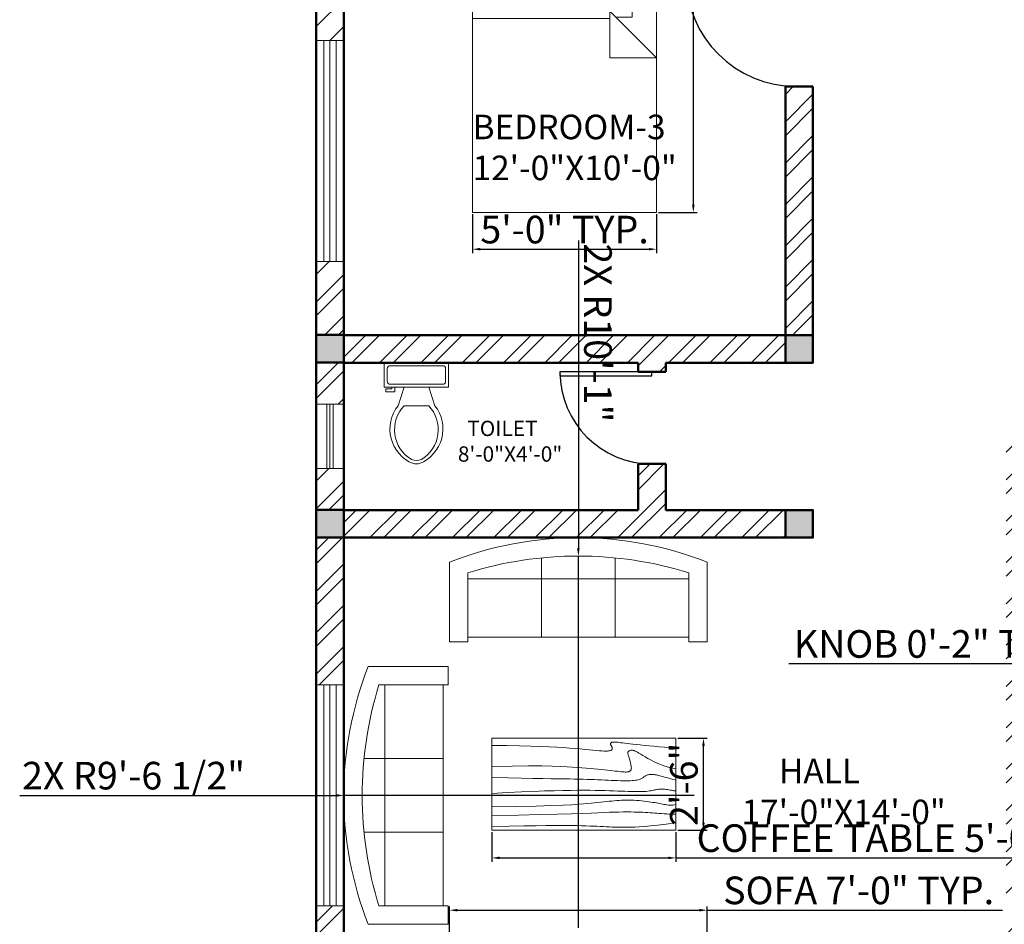
# Model space of a CAD drawing. Units: inches. Extents: x 381 to 1001, y 3003 to 3971.
# Tile 2 of 4: x 381 to 702, y 3347 to 3641. Entities that reach past the tile are written whole.
import ezdxf

# ---------------------------------------------------------------- set-up
doc = ezdxf.new("R2010")
doc.units = ezdxf.units.IN
for name, color, linetype, lineweight in [('A-ANNO-DIMS', 2, 'Continuous', 18), ('A-AREA-IDEN', 7, 'Continuous', 18), ('A-COLS', 7, 'Continuous', 50), ('A-DOOR', 4, 'Continuous', 25), ('A-FLOR-FIXT', 9, 'Continuous', 18), ('A-FURN', 8, 'Continuous', 18), ('A-GLAZ', 244, 'Continuous', 18), ('A-WALL', 7, 'Continuous', 50), ('A-WALL-PATT', 252, 'Continuous', 13)]:
    doc.layers.add(name, color=color, linetype=linetype, lineweight=lineweight)
doc.styles.get("Standard").update_dxf_attribs({"font": 'arial.ttf'})
doc.dimstyles.new('ISO-25', dxfattribs={"dimtxt": 9, "dimasz": 2.5, "dimexe": 1.25, "dimexo": 0.625, "dimtad": 1, "dimlunit": 3, "dimtxsty": 'Standard', "dimcen": 2.5, "dimadec": 0, "dimazin": 0, "dimtfac": 1, "dimtmove": 0, "dimatfit": 3, "dimfxl": 1, "dimarcsym": 0})

# ---------------------------------------------------------------- blocks, each defined once
blk = doc.blocks.new('*U3')
for p, q in [((0, 0), (0, -6)), ((-40, 0), (-40, -6))]:
    blk.add_line(p, q)
blk.add_lwpolyline([(0, 0), (0, 40), (-1.75, 40), (-1.75, 0)], close=True)
blk.add_arc((0, 0), 40, 90, 180)
blk = doc.blocks.new('*U9')
for p, q in [((9.5, -6), (9.5, -2)), ((-10, -8.5), (-8, -8.5)), ((-10, -9.5), (-10, -8.5)), ((-7, -9.5), (-10, -9.5)), ((-8, -8.5), (-8, -8)), ((-7, -8), (-7, -9.5)), ((-4, -8), (-6, -14)), ((4, -8), (6, -14)), ((4, -14), (-4, -14))]:
    blk.add_line(p, q)
blk.add_lwpolyline([(10.5, -8), (10.5, 0), (-10.5, 0), (-10.5, -8)], close=True)
for points in [[(-9.5, -2), (-9.5, -6)], [(8.5, -1), (-8.5, -1)], [(-8.5, -7), (8.5, -7)]]:
    blk.add_lwpolyline(points)
for centre, radius, start, end in [((-8.62, -1.88), 0.884, 81.8699, 188.1301), ((8.62, -1.88), 0.884, 351.8699, 98.1301), ((-8.62, -6.12), 0.884, 171.8699, 278.1301), ((8.62, -6.12), 0.884, 261.8699, 8.1301), ((3.52, -21.58), 12.17, 141.4691, 247.9714), ((4.2, -21.82), 11.33, 136.3677, 238.9468), ((-3.52, -21.58), 12.17, 292.0284, 38.5307), ((-4.2, -21.82), 11.33, 301.053, 43.6321), ((0, -27.88), 4, 245.7318, 294.2682), ((0, -29), 4, 254.8605, 285.1395)]:
    blk.add_arc(centre, radius, start, end)
blk = doc.blocks.new('Bed - Queen')
for p, q in [((0, -80.00003), (0, 0)), ((0, 0), (59.99999, 0)), ((59.99999, 0), (59.99999, -80.00003)), ((7.99999, -1.2), (28.79998, -1.2)), ((7.99999, -14.4), (7.99999, -1.2)), ((28.79998, -1.2), (28.79998, -14.4)), ((31.19999, -1.2), (51.99999, -1.2)), ((31.19999, -14.4), (31.19999, -1.2)), ((51.99999, -1.2), (51.99999, -16.4)), ((0, -14.4), (44.8, -14.4)), ((59.99999, -29.6), (44.8, -14.4)), ((44.8, -14.4), (44.8, -29.6)), ((44.8, -16.8), (0, -16.8)), ((51.99999, -16.4), (46.79936, -16.4)), ((44.8, -29.6), (59.99999, -29.6)), ((59.99999, -80.00003), (0, -80.00003))]:
    blk.add_line(p, q)
blk = doc.blocks.new('Sofa - Roundback 7 ft.')
for p, q in [((-12.00002, -32.4421), (-12.00003, -6.5971)), ((11.99997, -32.4421), (11.99998, -6.5971)), ((-36.000027, -34), (-36.000027, -11.4696)), ((35.99998, -34), (35.99998, -11.4696)), ((-35.999844, -13.3819), (35.9998, -13.3819)), ((-36.000027, -32.4421), (35.99998, -32.4421))]:
    blk.add_line(p, q)
for points in [[(-36.000027, -34), (-42.000027, -34), (-42.000027, -8)], [(41.99998, -8), (41.99998, -34), (35.99998, -34)]]:
    blk.add_lwpolyline(points)
for centre, radius, start, end in [((0, -114.25), 114.25, 68.43141, 111.5686), ((-0.00001, -127.1968), 121.1968, 72.72033, 107.2797)]:
    blk.add_arc(centre, radius, start, end)
blk = doc.blocks.new('Table - Rectangular Woodgrain 60 x 30 in.')
for p, q in [((0, 0), (0, -30)), ((60, 0), (0, 0)), ((60, -30), (60, 0)), ((0, -30), (60, -30))]:
    blk.add_line(p, q)
for points in [[(0, -2.4), (4.8155, -2.418), (9.0302, -2.4688), (12.709, -2.5477), (15.9167, -2.65), (18.7181, -2.7711), (21.1781, -2.9063), (23.3616, -3.0508), (25.3333, -3.2), (27.1477, -3.3495), (28.8172, -3.4958), (30.3437, -3.636), (31.7291, -3.7667), (32.9756, -3.8849), (34.0849, -3.9875), (35.059, -4.0714), (35.9, -4.1334), (36.6114, -4.1711), (37.2041, -4.1854), (37.6906, -4.1779), (38.0833, -4.15), (38.3948, -4.1034), (38.6375, -4.0396), (38.8239, -3.9602), (38.9666, -3.8667), (39.0764, -3.7608), (39.1573, -3.6448), (39.2116, -3.521), (39.2416, -3.3917), (39.2498, -3.2593), (39.2385, -3.1261), (39.21, -2.9944), (39.1666, -2.8667), (39.111, -2.7447), (39.0468, -2.6281), (38.978, -2.5163), (38.9083, -2.4083), (38.8418, -2.3035), (38.7823, -2.201), (38.7337, -2.1001), (38.7, -2), (38.6844, -1.9003), (38.6875, -1.8021), (38.7094, -1.707), (38.75, -1.6167), (38.8094, -1.5326), (38.8875, -1.4563), (38.9844, -1.3893), (39.1, -1.3333), (39.2351, -1.2896), (39.3937, -1.2583), (39.5804, -1.2396), (39.8, -1.2333), (40.057, -1.2396), (40.3562, -1.2583), (40.7023, -1.2896), (41.1, -1.3333), (41.5547, -1.3895), (42.0755, -1.4573), (42.6721, -1.5361), (43.3542, -1.625), (44.1316, -1.7233), (45.014, -1.8302), (46.0114, -1.9449), (47.1333, -2.0667), (48.3862, -2.1947), (49.7625, -2.3281), (51.2513, -2.4663), (52.8416, -2.6083), (54.5226, -2.7535), (56.2833, -2.9011), (58.1127, -3.0501), (60, -3.2)], [(0, -9.2), (6.5759, -9.0858), (11.9385, -9.0365), (16.2527, -9.0418), (19.6833, -9.0917), (22.3952, -9.1759), (24.5531, -9.2844), (26.322, -9.4069), (27.8666, -9.5333), (29.3241, -9.6553), (30.7203, -9.7719), (32.0532, -9.8837), (33.3208, -9.9917), (34.5213, -10.0965), (35.6526, -10.199), (36.7128, -10.2999), (37.7, -10.4), (38.6129, -10.4996), (39.4531, -10.5969), (40.223, -10.6895), (40.925, -10.775), (41.5613, -10.8512), (42.1344, -10.9156), (42.6465, -10.966), (43.1, -11), (43.4976, -11.0158), (43.8437, -11.0136), (44.143, -10.9942), (44.4, -10.9583), (44.6195, -10.9069), (44.8062, -10.8406), (44.9648, -10.7603), (45.1, -10.6667), (45.2155, -10.5598), (45.3114, -10.4365), (45.3871, -10.2929), (45.4416, -10.125), (45.4743, -9.929), (45.4844, -9.7011), (45.4709, -9.4371), (45.4333, -9.1333), (45.3716, -8.7883), (45.2896, -8.4104), (45.1919, -8.0107), (45.0833, -7.6), (44.9685, -7.1893), (44.8521, -6.7896), (44.7388, -6.4117), (44.6333, -6.0667), (44.54, -5.7628), (44.4614, -5.4979), (44.4001, -5.2675), (44.3583, -5.0667), (44.3384, -4.8909), (44.3427, -4.7354), (44.3736, -4.5956), (44.4333, -4.4667), (44.5236, -4.3453), (44.6427, -4.2333), (44.7884, -4.1339), (44.9583, -4.05), (45.1501, -3.9849), (45.3614, -3.9417), (45.59, -3.9234), (45.8333, -3.9333), (46.0915, -3.9749), (46.3734, -4.0531), (46.6906, -4.1736), (47.0542, -4.3417), (47.4756, -4.5629), (47.9661, -4.8427), (48.5372, -5.1866), (49.2, -5.6), (49.9676, -6.0844), (50.8594, -6.625), (51.8965, -7.2031), (53.1, -7.8), (54.491, -8.3969), (56.0906, -8.975), (57.9199, -9.5156), (60, -10)], [(0, -12.8), (5.1847, -12.9322), (9.6213, -13.0323), (13.3963, -13.1059), (16.5958, -13.1583), (19.3063, -13.1952), (21.614, -13.2219), (23.6054, -13.2439), (25.3666, -13.2667), (26.9728, -13.2947), (28.4531, -13.3281), (29.8256, -13.3663), (31.1083, -13.4083), (32.3191, -13.4535), (33.476, -13.501), (34.597, -13.5501), (35.7, -13.6), (36.7984, -13.6497), (37.8875, -13.6979), (38.9578, -13.743), (40, -13.7833), (41.0047, -13.8174), (41.9625, -13.8438), (42.864, -13.8607), (43.7, -13.8667), (44.4631, -13.8604), (45.1552, -13.8417), (45.7801, -13.8104), (46.3416, -13.7667), (46.8439, -13.7104), (47.2906, -13.6417), (47.6858, -13.5604), (48.0333, -13.4667), (48.3375, -13.3608), (48.6042, -13.2448), (48.8396, -13.121), (49.05, -12.9917), (49.2417, -12.8593), (49.4208, -12.7261), (49.5937, -12.5944), (49.7667, -12.4667), (49.9452, -12.3451), (50.1323, -12.2313), (50.3303, -12.1268), (50.5416, -12.0333), (50.7686, -11.9524), (51.0135, -11.8854), (51.2788, -11.8341), (51.5666, -11.8), (51.8785, -11.7843), (52.2116, -11.7865), (52.562, -11.8059), (52.926, -11.8417), (53.2998, -11.8931), (53.6795, -11.9594), (54.0614, -12.0397), (54.4416, -12.1333), (54.8223, -12.2401), (55.2293, -12.3625), (55.6942, -12.5037), (56.2489, -12.6667), (56.9251, -12.8547), (57.7545, -13.0708), (58.7689, -13.3182), (60, -13.6)], [(0, -18), (5.124, -17.7273), (9.6609, -17.5057), (13.6705, -17.3303), (17.2125, -17.1958), (20.3467, -17.0973), (23.1328, -17.0297), (25.6307, -16.9878), (27.9, -16.9667), (29.9928, -16.9617), (31.9302, -16.9703), (33.7254, -16.9907), (35.3917, -17.0208), (36.9423, -17.0588), (38.3906, -17.1026), (39.7499, -17.1503), (41.0333, -17.2), (42.2519, -17.2496), (43.4073, -17.2969), (44.4986, -17.3395), (45.525, -17.375), (46.4858, -17.4012), (47.3802, -17.4156), (48.2074, -17.416), (48.9667, -17.4), (49.6583, -17.3662), (50.2872, -17.3167), (50.8595, -17.2547), (51.3812, -17.1833), (51.8584, -17.1057), (52.2971, -17.025), (52.7034, -16.9443), (53.0833, -16.8667), (53.443, -16.7951), (53.789, -16.7313), (54.128, -16.6768), (54.4666, -16.6334), (54.8115, -16.6024), (55.1693, -16.5854), (55.5465, -16.5841), (55.95, -16.6), (56.3828, -16.6337), (56.8346, -16.6823), (57.2915, -16.7418), (57.7396, -16.8084), (58.165, -16.878), (58.5539, -16.9469), (58.8924, -17.0111), (59.1666, -17.0667), (59.3679, -17.1107), (59.5078, -17.1438), (59.6032, -17.1675), (59.6708, -17.1833), (59.7275, -17.193), (59.7901, -17.1979), (59.8753, -17.1998), (60, -17.2)], [(0, -22.4), (8.0098, -22.2501), (14.4094, -22.1011), (19.4168, -21.9535), (23.25, -21.8083), (26.1269, -21.6663), (28.2656, -21.5281), (29.884, -21.3947), (31.2, -21.2667), (32.3967, -21.1448), (33.5172, -21.0292), (34.5697, -20.9198), (35.5625, -20.8167), (36.5037, -20.7198), (37.4015, -20.6292), (38.2642, -20.5448), (39.1, -20.4667), (39.9164, -20.3951), (40.7187, -20.3313), (41.5117, -20.2768), (42.3, -20.2333), (43.0883, -20.2024), (43.8812, -20.1854), (44.6836, -20.1841), (45.5, -20.2), (46.3328, -20.234), (47.1747, -20.2844), (48.0163, -20.3488), (48.8479, -20.425), (49.66, -20.5106), (50.4429, -20.6031), (51.1872, -20.7004), (51.8833, -20.8), (52.5246, -20.8999), (53.1166, -20.9995), (53.6681, -21.0983), (54.1875, -21.1958), (54.6834, -21.2919), (55.1646, -21.3859), (55.6394, -21.4777), (56.1167, -21.5667), (56.6028, -21.6515), (57.0961, -21.7266), (57.5929, -21.7852), (58.0896, -21.8208), (58.5823, -21.8268), (59.0674, -21.7964), (59.5412, -21.723), (60, -21.6)], [(0, -25.2), (8.6355, -25.0504), (15.7026, -24.9031), (21.4049, -24.7606), (25.9458, -24.625), (29.529, -24.4988), (32.3578, -24.3844), (34.6359, -24.284), (36.5667, -24.2), (38.3213, -24.1341), (39.9417, -24.0854), (41.437, -24.0523), (42.8167, -24.0333), (44.0901, -24.0268), (45.2667, -24.0313), (46.3557, -24.0451), (47.3667, -24.0667), (48.309, -24.0947), (49.1928, -24.1287), (50.0284, -24.168), (50.826, -24.2125), (51.5959, -24.2617), (52.3483, -24.3151), (53.0935, -24.3725), (53.8417, -24.4334), (54.6009, -24.497), (55.3699, -24.561), (56.1454, -24.6226), (56.9239, -24.6792), (57.7021, -24.7279), (58.4764, -24.7662), (59.2435, -24.7911), (60, -24.8)], [(0, -28.8), (5.6867, -28.6681), (10.45, -28.5698), (14.407, -28.5012), (17.675, -28.4584), (20.3711, -28.4374), (22.6125, -28.4344), (24.5164, -28.4455), (26.2, -28.4667), (27.762, -28.4947), (29.2276, -28.5281), (30.6033, -28.5663), (31.8958, -28.6084), (33.1118, -28.6535), (34.2578, -28.7011), (35.3405, -28.7501), (36.3666, -28.8), (37.3443, -28.8497), (38.288, -28.8974), (39.2137, -28.9412), (40.1375, -28.9792), (41.0753, -29.0093), (42.0432, -29.0297), (43.0572, -29.0384), (44.1333, -29.0333), (45.2936, -29.0114), (46.5843, -28.9641), (48.0579, -28.8816), (49.7666, -28.7542), (51.7629, -28.5721), (54.0989, -28.3255), (56.8272, -28.0048), (60, -27.6)]]:
    blk.add_lwpolyline(points)
blk = doc.blocks.new('WIN-72X9')
for p, q in [((72, 6.5), (0, 6.5)), ((72, 4.5), (0, 4.5)), ((72, 2.5), (0, 2.5))]:
    blk.add_line(p, q)
blk.add_lwpolyline([(72, 9), (72, 0), (0, 0), (0, 9)], close=True)
blk = doc.blocks.new('VENT-WIN-21X9')
for p, q in [((3.5, 0), (3.5, 21)), ((4.5, 0), (4.5, 21)), ((5.5, 0), (5.5, 21))]:
    blk.add_line(p, q)
blk.add_lwpolyline([(9, 21), (9, 0), (0, 0), (0, 21)], close=True)
blk = doc.blocks.new('COLUMN-9X9')
h = blk.add_hatch(color=256)
h.dxf.hatch_style = 1
h.paths.add_polyline_path([(9, 9), (0, 9), (0, 0), (9, 0)])
blk.add_lwpolyline([(0, 9), (9, 9), (9, 0), (0, 0)], close=True)
blk = doc.blocks.new('*D36')
at = {"layer": 'A-ANNO-DIMS', "color": 0, "lineweight": -2, "transparency": 16777216}
for p, q in [((601.08, 3658.56), (601.08, 3794.71)), ((589.7, 3658.56), (602.33, 3658.56)), ((601.08, 3581.06), (601.08, 3656.06)), ((589.7, 3578.56), (602.33, 3578.56))]:
    blk.add_line(p, q, dxfattribs=at)
at = {"layer": 'A-ANNO-DIMS', "color": 0, "transparency": 16777216}
for points in [[(600.66, 3656.06), (601.49, 3656.06), (601.08, 3658.56)], [(600.66, 3581.06), (601.49, 3581.06), (601.08, 3578.56)]]:
    blk.add_solid(points, dxfattribs=at)
at = {"layer": 'Defpoints', "color": 0, "transparency": 16777216}
for p in [(589.08, 3658.56), (601.08, 3658.56), (589.08, 3578.56)]:
    blk.add_point(p, dxfattribs=at)
at = {"layer": 'A-ANNO-DIMS', "color": 0, "transparency": 16777216, "insert": (595.52, 3727.89), "char_height": 9, "attachment_point": 5, "rotation": 90}
blk.add_mtext('QUEEN BED 6\'-8" TYP.', dxfattribs=at)
blk = doc.blocks.new('*D37')
at = {"layer": 'A-ANNO-DIMS', "color": 0, "lineweight": -2, "transparency": 16777216}
for p, q in [((529.08, 3577.94), (529.08, 3565.31)), ((589.08, 3577.94), (589.08, 3565.31)), ((531.58, 3566.56), (586.58, 3566.56))]:
    blk.add_line(p, q, dxfattribs=at)
at = {"layer": 'A-ANNO-DIMS', "color": 0, "transparency": 16777216}
for points in [[(531.58, 3566.98), (531.58, 3566.15), (529.08, 3566.56)], [(586.58, 3566.98), (586.58, 3566.15), (589.08, 3566.56)]]:
    blk.add_solid(points, dxfattribs=at)
at = {"layer": 'Defpoints', "color": 0, "transparency": 16777216}
for p in [(529.08, 3578.56), (589.08, 3578.56), (589.08, 3566.56)]:
    blk.add_point(p, dxfattribs=at)
at = {"layer": 'A-ANNO-DIMS', "color": 0, "transparency": 16777216, "insert": (559.08, 3571.79), "char_height": 9, "attachment_point": 5}
blk.add_mtext('5\'-0" TYP.', dxfattribs=at)
blk = doc.blocks.new('*D38')
at = {"layer": 'A-ANNO-DIMS', "color": 0, "lineweight": -2, "transparency": 16777216}
for p, q in [((521.58, 3339.19), (521.58, 3352.41)), ((605.58, 3339.19), (605.58, 3352.41)), ((524.08, 3351.16), (603.08, 3351.16)), ((605.58, 3351.16), (701.87, 3351.16))]:
    blk.add_line(p, q, dxfattribs=at)
at = {"layer": 'A-ANNO-DIMS', "color": 0, "transparency": 16777216}
for points in [[(524.08, 3351.58), (524.08, 3350.75), (521.58, 3351.16)], [(603.08, 3351.58), (603.08, 3350.75), (605.58, 3351.16)]]:
    blk.add_solid(points, dxfattribs=at)
at = {"layer": 'Defpoints', "color": 0, "transparency": 16777216}
for p in [(605.58, 3351.16), (521.58, 3338.56), (605.58, 3338.56)]:
    blk.add_point(p, dxfattribs=at)
at = {"layer": 'A-ANNO-DIMS', "color": 0, "transparency": 16777216, "insert": (654.97, 3356.45), "char_height": 9, "attachment_point": 5}
blk.add_mtext('SOFA 7\'-0" TYP.', dxfattribs=at)
blk = doc.blocks.new('*D46')
at = {"layer": 'A-ANNO-DIMS', "color": 0, "lineweight": -2, "transparency": 16777216}
for p, q in [((732.1, 3431.81), (732.1, 3432.72)), ((733.98, 3431.81), (733.98, 3432.72)), ((729.6, 3431.47), (632.26, 3431.47)), ((733.98, 3431.47), (732.1, 3431.47)), ((736.48, 3431.47), (738.98, 3431.47))]:
    blk.add_line(p, q, dxfattribs=at)
at = {"layer": 'A-ANNO-DIMS', "color": 0, "transparency": 16777216}
for points in [[(729.6, 3431.88), (729.6, 3431.05), (732.1, 3431.47)], [(736.48, 3431.88), (736.48, 3431.05), (733.98, 3431.47)]]:
    blk.add_solid(points, dxfattribs=at)
at = {"layer": 'Defpoints', "color": 0, "transparency": 16777216}
for p in [(732.1, 3431.47), (732.1, 3431.18), (733.98, 3431.18)]:
    blk.add_point(p, dxfattribs=at)
at = {"layer": 'A-ANNO-DIMS', "color": 0, "transparency": 16777216, "insert": (679.68, 3436.75), "char_height": 9, "attachment_point": 5}
blk.add_mtext('KNOB 0\'-2" TYP.', dxfattribs=at)
blk = doc.blocks.new('*D50')
at = {"layer": 'A-ANNO-DIMS', "color": 0, "lineweight": -2, "transparency": 16777216}
for p, q in [((535.37, 3376.58), (535.37, 3366.95)), ((595.37, 3376.58), (595.37, 3366.95)), ((537.87, 3368.2), (592.87, 3368.2)), ((595.37, 3368.2), (720.75, 3368.2))]:
    blk.add_line(p, q, dxfattribs=at)
at = {"layer": 'A-ANNO-DIMS', "color": 0, "transparency": 16777216}
for points in [[(537.87, 3368.62), (537.87, 3367.79), (535.37, 3368.2)], [(592.87, 3368.62), (592.87, 3367.79), (595.37, 3368.2)]]:
    blk.add_solid(points, dxfattribs=at)
at = {"layer": 'Defpoints', "color": 0, "transparency": 16777216}
for p in [(535.37, 3377.2), (595.37, 3377.2), (595.37, 3368.2)]:
    blk.add_point(p, dxfattribs=at)
at = {"layer": 'A-ANNO-DIMS', "color": 0, "transparency": 16777216, "insert": (659.31, 3373.48), "char_height": 9, "attachment_point": 5}
blk.add_mtext('COFFEE TABLE 5\'-0"', dxfattribs=at)
blk = doc.blocks.new('*D51')
at = {"layer": 'A-ANNO-DIMS', "color": 0, "lineweight": -2, "transparency": 16777216}
for p, q in [((595.99, 3407.2), (605.62, 3407.2)), ((604.37, 3379.7), (604.37, 3404.7)), ((595.99, 3377.2), (605.62, 3377.2))]:
    blk.add_line(p, q, dxfattribs=at)
at = {"layer": 'A-ANNO-DIMS', "color": 0, "transparency": 16777216}
for points in [[(603.95, 3404.7), (604.79, 3404.7), (604.37, 3407.2)], [(603.95, 3379.7), (604.79, 3379.7), (604.37, 3377.2)]]:
    blk.add_solid(points, dxfattribs=at)
at = {"layer": 'Defpoints', "color": 0, "transparency": 16777216}
for p in [(595.37, 3407.2), (604.37, 3407.2), (595.37, 3377.2)]:
    blk.add_point(p, dxfattribs=at)
at = {"layer": 'A-ANNO-DIMS', "color": 0, "transparency": 16777216, "insert": (599.15, 3392.2), "char_height": 9, "attachment_point": 5, "rotation": 90}
blk.add_mtext('2\'-6"', dxfattribs=at)
blk = doc.blocks.new('*D61')
at = {"layer": 'A-ANNO-DIMS', "color": 0, "lineweight": -2, "transparency": 16777216}
for p, q in [((563.58, 3569.42), (563.58, 3469.06)), ((563.58, 3345.37), (563.58, 3466.56))]:
    blk.add_line(p, q, dxfattribs=at)
at = {"layer": 'A-ANNO-DIMS', "color": 0, "transparency": 16777216}
blk.add_solid([(563.99, 3469.06), (563.16, 3469.06), (563.58, 3466.56)], dxfattribs=at)
at = {"layer": 'Defpoints', "color": 0, "transparency": 16777216}
for p in [(563.58, 3466.56), (563.58, 3345.37)]:
    blk.add_point(p, dxfattribs=at)
at = {"layer": 'A-ANNO-DIMS', "color": 0, "transparency": 16777216, "insert": (568.8, 3539.28), "char_height": 9, "attachment_point": 5, "rotation": 270.0001}
blk.add_mtext('2X R10\'-1"', dxfattribs=at)
blk = doc.blocks.new('*D62')
at = {"layer": 'A-ANNO-DIMS', "color": 0, "lineweight": -2, "transparency": 16777216}
for p, q in [((381.4, 3388.56), (484.58, 3388.56)), ((601.33, 3388.56), (487.08, 3388.56))]:
    blk.add_line(p, q, dxfattribs=at)
at = {"layer": 'A-ANNO-DIMS', "color": 0, "transparency": 16777216}
blk.add_solid([(484.58, 3388.98), (484.58, 3388.15), (487.08, 3388.56)], dxfattribs=at)
at = {"layer": 'Defpoints', "color": 0, "transparency": 16777216}
for p in [(487.08, 3388.56), (601.33, 3388.56)]:
    blk.add_point(p, dxfattribs=at)
at = {"layer": 'A-ANNO-DIMS', "color": 0, "transparency": 16777216, "insert": (418.53, 3393.84), "char_height": 9, "attachment_point": 5}
blk.add_mtext('2X R9\'-6 1/2"', dxfattribs=at)

msp = doc.modelspace()

# ---------------------------------------------------------------- hatches: boundary and pattern name
at = {"layer": 'A-WALL-PATT'}
h = msp.add_hatch(dxfattribs=at)
h.set_pattern_fill('ANSI32', color=256)
h.paths.add_polyline_path([(652.078, 3667.565), (487.078, 3667.565), (487.078, 3658.565), (631.078, 3658.565), (631.078, 3655.565), (634.678, 3655.565), (640.078, 3655.565), (640.078, 3658.565), (652.078, 3658.565)])
h.paths.add_polyline_path([(487.078, 3658.637), (478.078, 3658.637), (478.078, 3634.565), (487.078, 3634.565)])
h.paths.add_polyline_path([(487.078, 3703.565), (478.078, 3703.565), (478.078, 3667.637), (487.078, 3667.637)])
h.paths.add_polyline_path([(661.078, 3811.637), (652.078, 3811.637), (652.078, 3706.565), (661.078, 3706.565)])
h.paths.add_polyline_path([(661.078, 3670.565), (655.678, 3670.565), (652.078, 3670.565), (652.078, 3667.637), (661.078, 3667.637)])
h.paths.add_polyline_path([(487.078, 3811.637), (478.078, 3811.637), (478.078, 3775.565), (487.078, 3775.565)])
h.paths.add_polyline_path([(487.078, 3880.565), (478.078, 3880.565), (478.078, 3820.637), (487.078, 3820.637)])
h.paths.add_polyline_path([(661.078, 3880.637), (652.078, 3880.637), (652.078, 3820.637), (661.078, 3820.637)])
h.paths.add_polyline_path([(652.078, 3820.565), (568.078, 3820.565), (568.078, 3823.565), (563.578, 3823.565), (562.078, 3823.565), (562.078, 3820.565), (559.078, 3820.565), (559.078, 3811.565), (652.078, 3811.565), (652.078, 3811.637)])
h.paths.add_polyline_path([(523.078, 3820.565), (487.078, 3820.565), (487.078, 3811.565), (523.078, 3811.565)])
h.paths.add_polyline_path([(619.798, 3889.565), (487.078, 3889.565), (487.078, 3880.565), (562.078, 3880.565), (562.078, 3853.565), (568.078, 3853.565), (568.078, 3880.565), (619.798, 3880.565)])
h.paths.add_polyline_path([(652.078, 3889.565), (640.798, 3889.565), (640.798, 3880.565), (652.078, 3880.565), (652.078, 3880.637)])
h.paths.add_polyline_path([(757.078, 3889.565), (661.078, 3889.565), (661.078, 3880.565), (757.078, 3880.565)])
h.paths.add_polyline_path([(766.078, 3880.637), (757.078, 3880.637), (757.078, 3820.637), (766.078, 3820.637)])
h.paths.add_polyline_path([(773.578, 3889.565), (766.078, 3889.565), (766.078, 3880.565), (773.578, 3880.565)])
h.paths.add_polyline_path([(931.078, 3889.565), (794.578, 3889.565), (794.578, 3880.565), (850.078, 3880.565), (850.078, 3853.565), (856.078, 3853.565), (856.078, 3880.565), (931.078, 3880.565)])
h.paths.add_polyline_path([(859.078, 3820.565), (856.078, 3820.565), (856.078, 3823.565), (850.078, 3823.565), (850.078, 3820.565), (766.078, 3820.565), (766.078, 3811.565), (859.078, 3811.565)])
h.paths.add_polyline_path([(940.078, 3880.637), (931.078, 3880.637), (931.078, 3820.637), (940.078, 3820.637)])
h.paths.add_polyline_path([(931.078, 3820.565), (895.078, 3820.565), (895.078, 3811.565), (931.078, 3811.565)])
h.paths.add_polyline_path([(940.078, 3811.637), (931.078, 3811.637), (931.078, 3775.565), (940.078, 3775.565)])
h.paths.add_polyline_path([(766.078, 3811.637), (757.078, 3811.637), (757.078, 3706.565), (766.078, 3706.565)])
h.paths.add_polyline_path([(940.078, 3703.565), (931.078, 3703.565), (931.078, 3667.637), (940.078, 3667.637)])
h.paths.add_polyline_path([(931.078, 3667.565), (766.078, 3667.565), (766.078, 3658.565), (931.078, 3658.565)])
h.paths.add_polyline_path([(940.078, 3658.637), (931.078, 3658.637), (931.078, 3621.065), (940.078, 3621.065)])
h.paths.add_polyline_path([(940.078, 3549.065), (931.078, 3549.065), (931.078, 3511.637), (940.078, 3511.637)])
h.paths.add_polyline_path([(931.078, 3511.565), (847.078, 3511.565), (847.078, 3502.565), (931.078, 3502.565)])
h.paths.add_polyline_path([(802.078, 3511.565), (712.078, 3511.565), (712.078, 3502.565), (802.078, 3502.565)])
h.paths.add_polyline_path([(712.078, 3502.637), (703.078, 3502.637), (703.078, 3355.637), (712.078, 3355.637)])
h.paths.add_polyline_path([(740.578, 3355.565), (712.078, 3355.565), (712.078, 3346.565), (740.578, 3346.565)])
h.paths.add_polyline_path([(841.078, 3355.565), (812.578, 3355.565), (812.578, 3346.565), (841.078, 3346.565)])
h.paths.add_polyline_path([(850.078, 3412.565), (841.078, 3412.565), (841.078, 3355.637), (850.078, 3355.637)], flags=17)
h.paths.add_polyline_path([(940.078, 3502.637), (931.078, 3502.637), (931.078, 3454.565), (841.078, 3454.565), (841.078, 3442.565), (850.078, 3442.565), (850.078, 3445.565), (931.078, 3445.565), (931.078, 3355.637), (940.078, 3355.637)])
h.paths.add_polyline_path([(931.078, 3355.565), (850.078, 3355.565), (850.078, 3346.565), (931.078, 3346.565)])
h.paths.add_polyline_path([(712.078, 3346.637), (703.078, 3346.637), (703.078, 3304.565), (700.078, 3304.565), (700.078, 3295.565), (712.078, 3295.565)])
h.paths.add_polyline_path([(622.078, 3202.565), (487.078, 3202.565), (487.078, 3193.565), (622.078, 3193.565)])
h.paths.add_polyline_path([(487.078, 3295.637), (478.078, 3295.637), (478.078, 3202.637), (487.078, 3202.637)])
h.paths.add_polyline_path([(712.078, 3295.565), (703.078, 3295.565), (703.078, 3202.565), (712.078, 3202.565)])
h = msp.add_hatch(dxfattribs=at)
h.set_pattern_fill('ANSI32', color=256)
h.paths.add_polyline_path([(487.078, 3352.565), (478.078, 3352.565), (478.078, 3304.637), (487.078, 3304.637)])
h.paths.add_polyline_path([(631.078, 3304.565), (487.078, 3304.565), (487.078, 3295.565), (631.078, 3295.565)])
h.paths.add_polyline_path([(487.078, 3472.637), (478.078, 3472.637), (478.078, 3424.565), (487.078, 3424.565)])
h.paths.add_polyline_path([(631.078, 3481.565), (592.078, 3481.565), (592.078, 3496.565), (583.078, 3496.565), (583.078, 3481.565), (487.078, 3481.565), (487.078, 3472.565), (631.078, 3472.565)])
h.paths.add_polyline_path([(487.078, 3562.565), (478.078, 3562.565), (478.078, 3538.637), (487.078, 3538.637)])
h.paths.add_polyline_path([(487.078, 3529.637), (478.078, 3529.637), (478.078, 3516.065), (487.078, 3516.065)])
h.paths.add_polyline_path([(487.078, 3495.065), (478.078, 3495.065), (478.078, 3481.637), (487.078, 3481.637)])
h.paths.add_polyline_path([(631.078, 3538.565), (487.078, 3538.565), (487.078, 3529.565), (583.078, 3529.565), (583.078, 3526.565), (587.578, 3526.565), (592.078, 3526.565), (592.078, 3529.565), (631.078, 3529.565)])
h.paths.add_polyline_path([(640.078, 3619.565), (631.078, 3619.565), (631.078, 3538.565), (640.078, 3538.565)])

# ---------------------------------------------------------------- linework, layer by layer
at = {"layer": 'A-WALL'}
for p, q in [((478.078, 3889.565), (478.078, 3193.565)), ((487.078, 3658.565), (487.078, 3538.565)), ((631.078, 3619.565), (640.078, 3619.565)), ((631.078, 3619.565), (631.078, 3538.565)), ((640.078, 3619.565), (640.078, 3529.565)), ((487.078, 3538.565), (631.078, 3538.565)), ((487.078, 3529.565), (583.078, 3529.565)), ((487.078, 3529.565), (487.078, 3481.565)), ((583.078, 3529.565), (583.078, 3526.565)), ((592.078, 3529.565), (592.078, 3526.565)), ((592.078, 3529.565), (640.078, 3529.565)), ((583.078, 3526.565), (592.078, 3526.565)), ((583.078, 3496.565), (592.078, 3496.565)), ((583.078, 3496.565), (583.078, 3481.565)), ((592.078, 3496.565), (592.078, 3481.565)), ((487.078, 3481.565), (583.078, 3481.565)), ((592.078, 3481.565), (640.078, 3481.565)), ((640.078, 3481.565), (640.078, 3472.565)), ((487.078, 3472.565), (640.078, 3472.565)), ((487.078, 3472.565), (487.078, 3304.565))]:
    msp.add_line(p, q, dxfattribs=at)

# ---------------------------------------------------------------- block references
at = {"layer": 'A-COLS'}
for p in [(478.078, 3529.637), (631.078, 3529.565), (478.078, 3472.637), (631.078, 3472.565)]:
    msp.add_blockref('COLUMN-9X9', p, dxfattribs=at)
at = {"layer": 'A-DOOR', "rotation": 90}
for p, xscale, yscale, zscale in [((634.678, 3655.565), 0.9, 0.9, 0.9), ((587.578, 3526.565), 0.75, 0.75, 0.75)]:
    msp.add_blockref('*U3', p, dxfattribs=dict(at, xscale=xscale, yscale=yscale, zscale=zscale))
at = {"layer": 'A-FLOR-FIXT'}
msp.add_blockref('*U9', (510.768, 3529.565), dxfattribs=at)
at = {"layer": 'A-FURN'}
for name, p in [('Bed - Queen', (529.078, 3658.565)), ('Sofa - Roundback 7 ft.', (563.578, 3472.565)), ('Table - Rectangular Woodgrain 60 x 30 in.', (535.37, 3407.202))]:
    msp.add_blockref(name, p, dxfattribs=at)
at = {"layer": 'A-FURN', "rotation": 89.99998708239097}
msp.add_blockref('Sofa - Roundback 7 ft.', (487.078, 3388.565), dxfattribs=at)
at = {"layer": 'A-GLAZ', "rotation": 90.00000000000011}
for p in [(487.078, 3562.565), (487.078, 3352.565)]:
    msp.add_blockref('WIN-72X9', p, dxfattribs=at)
at = {"layer": 'A-GLAZ'}
msp.add_blockref('VENT-WIN-21X9', (478.078, 3495.065), dxfattribs=at)

# ---------------------------------------------------------------- texts
at = {"layer": 'A-AREA-IDEN', "attachment_point": 1}
for s, width, insert, char_height in [('BEDROOM-3\\P12\'-0"X10\'-0"', 69.00419, (529.078, 3610.394), 8), ('  TOILET\\P8\'-0"X4\'-0"', 32.42882, (524.288, 3510.656), 5), ('     HALL\\P17\'-0"X14\'-0"', 64.05626, (616.792, 3400.516), 8)]:
    msp.add_mtext_dynamic_manual_height_columns(s, width=width, gutter_width=12.5, heights=[0], dxfattribs=dict(at, insert=insert, char_height=char_height))

# ---------------------------------------------------------------- dimensions: what is measured, and where the dimension line sits
at = {"layer": 'A-ANNO-DIMS'}
for base, p1, p2, angle, text, picture, middle in [((601.078, 3658.565), (589.078, 3578.565), (589.078, 3658.565), 90, 'QUEEN BED <> TYP.', '*D36', (595.524, 3727.885)), ((732.098, 3431.466), (733.977, 3431.184), (732.098, 3431.184), 180, 'KNOB <> TYP.', '*D46', (679.68, 3436.748))]:
    dim = msp.add_linear_dim(base=base, p1=p1, p2=p2, angle=angle, text=text, dimstyle='ISO-25', override={"dimdec": 1, "dimlfac": 1, "dimrnd": 0, "dimzin": 1, "dimdsep": 46, "dimlunit": 4, "dimfrac": 2}, dxfattribs=at)
    dim.commit()
    dim.dimension.update_dxf_attribs({"geometry": picture, "text_midpoint": middle})
for base, p1, p2, text, picture, middle in [((589.078, 3566.565), (529.078, 3578.565), (589.078, 3578.565), '<> TYP.', '*D37', (559.078, 3571.785)), ((595.37, 3368.202), (535.37, 3377.202), (595.37, 3377.202), 'COFFEE TABLE <>', '*D50', (659.309, 3373.483)), ((605.578, 3351.165), (521.578, 3338.565), (605.578, 3338.565), 'SOFA <> TYP.', '*D38', (654.974, 3356.446))]:
    dim = msp.add_linear_dim(base=base, p1=p1, p2=p2, text=text, dimstyle='ISO-25', override={"dimdec": 1, "dimlfac": 1, "dimrnd": 0, "dimzin": 1, "dimdsep": 46, "dimlunit": 4, "dimfrac": 2}, dxfattribs=at)
    dim.commit()
    dim.dimension.update_dxf_attribs({"geometry": picture, "text_midpoint": middle})
for center, mpoint, picture, middle in [((563.578, 3345.368), (563.578, 3466.565), '*D61', (563.578, 3539.283)), ((601.328304, 3388.564916), (487.078304, 3388.565), '*D62', (418.528304, 3388.565))]:
    dim = msp.add_radius_dim(center=center, mpoint=mpoint, text='2X <>', dimstyle='ISO-25', override={"dimdec": 1, "dimlfac": 1, "dimrnd": 0, "dimzin": 1, "dimdsep": 46, "dimlunit": 4, "dimfrac": 2}, dxfattribs=at)
    dim.commit()
    dim.dimension.update_dxf_attribs({"geometry": picture, "text_midpoint": middle, "dimtype": 164})
dim = msp.add_linear_dim(base=(604.37, 3407.202), p1=(595.37, 3377.202), p2=(595.37, 3407.202), angle=90, dimstyle='ISO-25', override={"dimdec": 1, "dimlfac": 1, "dimrnd": 0, "dimzin": 1, "dimdsep": 46, "dimlunit": 4, "dimfrac": 2}, dxfattribs=at)
dim.commit()
dim.dimension.update_dxf_attribs({"geometry": '*D51', "text_midpoint": (599.149, 3392.202)})

doc.saveas('drawing.dxf')
